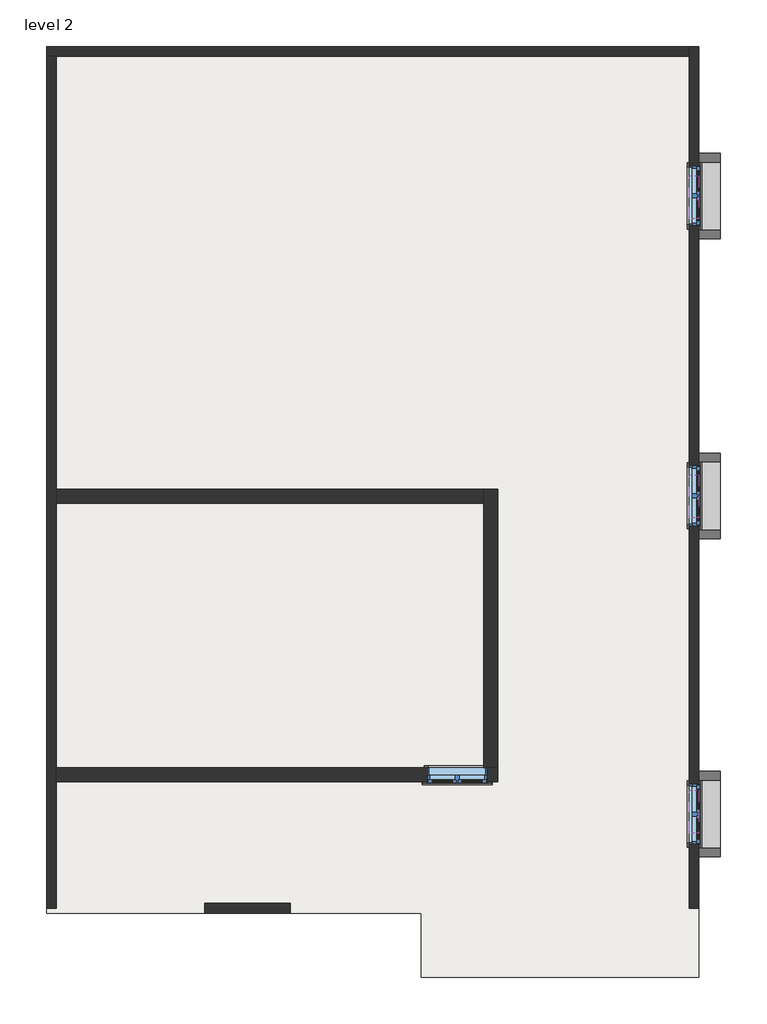
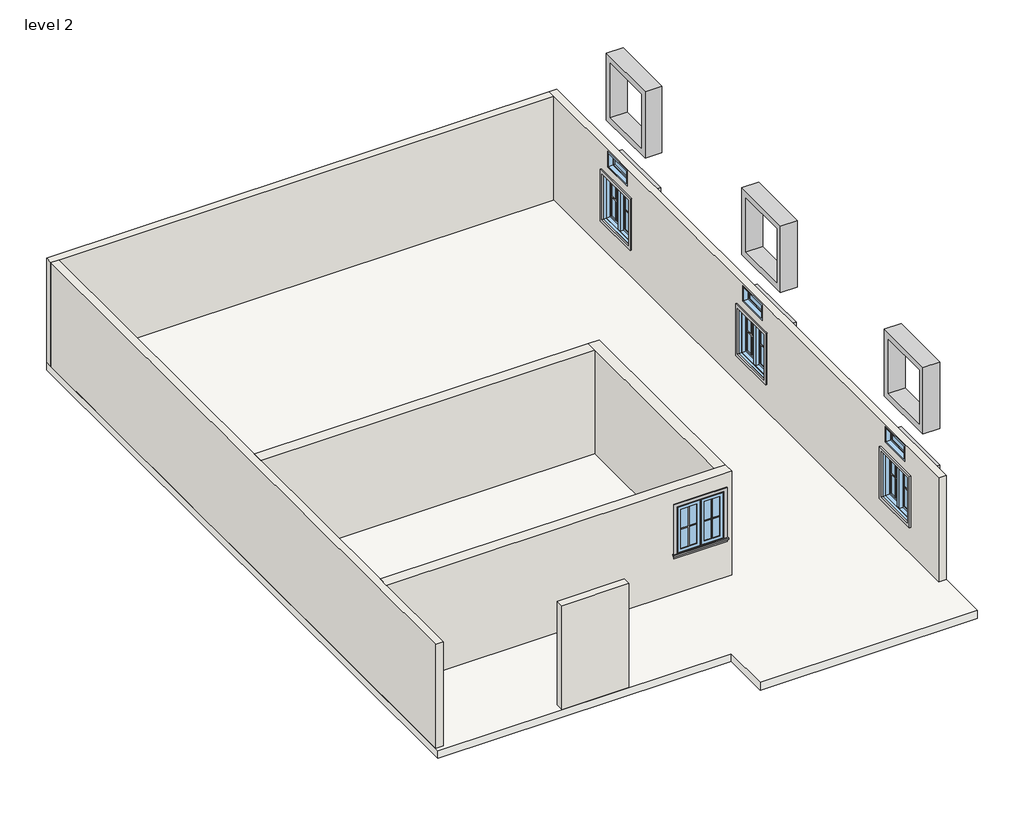
# One storey, incomplete: 16 proxies, 7 walls, 7 windows, 1 duct fitting, 1 slab.
"""IFC4 building model written with IfcOpenShell, lengths in millimetres."""

from ifc_helpers import new_model, si_unit, frame, origin, place, context, project, spatial, polyline, outline, extrude, faceted_brep, transform, mapped, element, save
from components import m_muntin_pattern_2x2_m_muntin_pattern_2x2_62480ac4, m_muntin_pattern_2x2_m_muntin_pattern_2x2_4fd78f17, m_trim_window_exterior_flat_with_sill_90d3a428, m_trim_window_interior_flat_picture_frame_6ca9b1f8, duct_fittings_2_duct_fittings_2_84becefd, m_fixed_0406_x_0610mm_8d3231a3, m_window_casement_double_850_x_900mm_0f766704, m_window_casement_double_850_x_900mm_77c4388a

model = new_model("IFC4")

# Units and contexts
model_context = context("Model", 3, world=origin())
ifc_project = project(units=[si_unit("LENGTHUNIT", "METRE", prefix="MILLI")], contexts=[model_context])

# Site, building, storey
site = spatial("IfcSite", under=ifc_project)
building = spatial("IfcBuilding", under=site)
storey = spatial("IfcBuildingStorey", under=building, Name="level 2", Elevation=5000.0)

# Proxies
placement = place(None, origin())
m_muntin_pattern_2x2_m_muntin_pattern_2x2_shape = m_muntin_pattern_2x2_m_muntin_pattern_2x2_62480ac4(model_context)
element("IfcBuildingElementProxy", 1, Name="M_Muntin Pattern_2x2 : M_Muntin Pattern_2x2", ObjectType="M_Muntin Pattern_2x2 : M_Muntin Pattern_2x2", at=placement, inside=storey, context=model_context, shape_type="MappedRepresentation", body=[
    mapped(m_muntin_pattern_2x2_m_muntin_pattern_2x2_shape, transform((-5582.3542042, -3112.6046146, 5837.792842), x_axis=(-1.0, 0.0, 0.0), y_axis=(0.0, -1.0, 0.0), z_axis=(0.0, 0.0, 1.0))),
])
element("IfcBuildingElementProxy", 2, Name="M_Muntin Pattern_2x2 : M_Muntin Pattern_2x2", ObjectType="M_Muntin Pattern_2x2 : M_Muntin Pattern_2x2", at=placement, inside=storey, context=model_context, shape_type="MappedRepresentation", body=[
    mapped(m_muntin_pattern_2x2_m_muntin_pattern_2x2_shape, transform((-2362.9917042, -3370.6171146, 5642.7567455), x_axis=(0.0, -1.0, 0.0), y_axis=(1.0, 0.0, 0.0), z_axis=(0.0, 0.0, 1.0))),
])
element("IfcBuildingElementProxy", 3, Name="M_Muntin Pattern_2x2 : M_Muntin Pattern_2x2", ObjectType="M_Muntin Pattern_2x2 : M_Muntin Pattern_2x2", at=placement, inside=storey, context=model_context, shape_type="MappedRepresentation", body=[
    mapped(m_muntin_pattern_2x2_m_muntin_pattern_2x2_shape, transform((-2362.9917042, 1160.7078854, 5642.7567455), x_axis=(0.0, -1.0, 0.0), y_axis=(1.0, 0.0, 0.0), z_axis=(0.0, 0.0, 1.0))),
])
element("IfcBuildingElementProxy", 4, Name="M_Muntin Pattern_2x2 : M_Muntin Pattern_2x2", ObjectType="M_Muntin Pattern_2x2 : M_Muntin Pattern_2x2", at=placement, inside=storey, context=model_context, shape_type="MappedRepresentation", body=[
    mapped(m_muntin_pattern_2x2_m_muntin_pattern_2x2_shape, transform((-2362.9917042, 5427.9078854, 5642.7567455), x_axis=(0.0, -1.0, 0.0), y_axis=(1.0, 0.0, 0.0), z_axis=(0.0, 0.0, 1.0))),
])
m_muntin_pattern_2x2_m_muntin_pattern_2x2_2_shape = m_muntin_pattern_2x2_m_muntin_pattern_2x2_4fd78f17(model_context)
element("IfcBuildingElementProxy", 5, Name="M_Muntin Pattern_2x2 : M_Muntin Pattern_2x2", ObjectType="M_Muntin Pattern_2x2 : M_Muntin Pattern_2x2", at=placement, inside=storey, context=model_context, shape_type="MappedRepresentation", body=[
    mapped(m_muntin_pattern_2x2_m_muntin_pattern_2x2_2_shape, transform((-6004.1792042, -3112.6046146, 5837.792842), x_axis=(1.0, 0.0, 0.0), y_axis=(0.0, 1.0, 0.0), z_axis=(0.0, 0.0, 1.0))),
])
element("IfcBuildingElementProxy", 6, Name="M_Muntin Pattern_2x2 : M_Muntin Pattern_2x2", ObjectType="M_Muntin Pattern_2x2 : M_Muntin Pattern_2x2", at=placement, inside=storey, context=model_context, shape_type="MappedRepresentation", body=[
    mapped(m_muntin_pattern_2x2_m_muntin_pattern_2x2_2_shape, transform((-2362.9917042, -3792.4421146, 5642.7567455), x_axis=(0.0, 1.0, 0.0), y_axis=(-1.0, 0.0, 0.0), z_axis=(0.0, 0.0, 1.0))),
])
element("IfcBuildingElementProxy", 7, Name="M_Muntin Pattern_2x2 : M_Muntin Pattern_2x2", ObjectType="M_Muntin Pattern_2x2 : M_Muntin Pattern_2x2", at=placement, inside=storey, context=model_context, shape_type="MappedRepresentation", body=[
    mapped(m_muntin_pattern_2x2_m_muntin_pattern_2x2_2_shape, transform((-2362.9917042, 738.8828854, 5642.7567455), x_axis=(0.0, 1.0, 0.0), y_axis=(-1.0, 0.0, 0.0), z_axis=(0.0, 0.0, 1.0))),
])
element("IfcBuildingElementProxy", 8, Name="M_Muntin Pattern_2x2 : M_Muntin Pattern_2x2", ObjectType="M_Muntin Pattern_2x2 : M_Muntin Pattern_2x2", at=placement, inside=storey, context=model_context, shape_type="MappedRepresentation", body=[
    mapped(m_muntin_pattern_2x2_m_muntin_pattern_2x2_2_shape, transform((-2362.9917042, 5006.0828854, 5642.7567455), x_axis=(0.0, 1.0, 0.0), y_axis=(-1.0, 0.0, 0.0), z_axis=(0.0, 0.0, 1.0))),
])
m_trim_window_exterior_flat_with_sill_shape = m_trim_window_exterior_flat_with_sill_90d3a428(model_context)
element("IfcBuildingElementProxy", 9, Name="M_Trim-Window-Exterior-Flat : with Sill", ObjectType="M_Trim-Window-Exterior-Flat : with Sill", at=placement, inside=storey, context=model_context, shape_type="MappedRepresentation", body=[
    mapped(m_trim_window_exterior_flat_with_sill_shape, transform((-5793.2667042, -3122.1296146, 6667.942842), x_axis=(1.0, 0.0, 0.0), y_axis=(0.0, 0.0, 1.0), z_axis=(0.0, -1.0, 0.0))),
])
element("IfcBuildingElementProxy", 10, Name="M_Trim-Window-Exterior-Flat : with Sill", ObjectType="M_Trim-Window-Exterior-Flat : with Sill", at=placement, inside=storey, context=model_context, shape_type="MappedRepresentation", body=[
    mapped(m_trim_window_exterior_flat_with_sill_shape, transform((-2353.4667042, -3581.5296146, 6472.9067455), x_axis=(0.0, 1.0, 0.0), y_axis=(0.0, 0.0, 1.0), z_axis=(1.0, 0.0, 0.0))),
])
element("IfcBuildingElementProxy", 11, Name="M_Trim-Window-Exterior-Flat : with Sill", ObjectType="M_Trim-Window-Exterior-Flat : with Sill", at=placement, inside=storey, context=model_context, shape_type="MappedRepresentation", body=[
    mapped(m_trim_window_exterior_flat_with_sill_shape, transform((-2353.4667042, 949.7953854, 6472.9067455), x_axis=(0.0, 1.0, 0.0), y_axis=(0.0, 0.0, 1.0), z_axis=(1.0, 0.0, 0.0))),
])
element("IfcBuildingElementProxy", 12, Name="M_Trim-Window-Exterior-Flat : with Sill", ObjectType="M_Trim-Window-Exterior-Flat : with Sill", at=placement, inside=storey, context=model_context, shape_type="MappedRepresentation", body=[
    mapped(m_trim_window_exterior_flat_with_sill_shape, transform((-2353.4667042, 5216.9953854, 6472.9067455), x_axis=(0.0, 1.0, 0.0), y_axis=(0.0, 0.0, 1.0), z_axis=(1.0, 0.0, 0.0))),
])
m_trim_window_interior_flat_picture_frame_shape = m_trim_window_interior_flat_picture_frame_6ca9b1f8(model_context)
element("IfcBuildingElementProxy", 13, Name="M_Trim-Window-Interior-Flat : Picture Frame", ObjectType="M_Trim-Window-Interior-Flat : Picture Frame", at=placement, inside=storey, context=model_context, shape_type="MappedRepresentation", body=[
    mapped(m_trim_window_interior_flat_picture_frame_shape, transform((-5793.2667042, -2922.1296146, 6667.942842), x_axis=(-1.0, 0.0, 0.0), y_axis=(0.0, 0.0, 1.0), z_axis=(0.0, 1.0, 0.0))),
])
element("IfcBuildingElementProxy", 14, Name="M_Trim-Window-Interior-Flat : Picture Frame", ObjectType="M_Trim-Window-Interior-Flat : Picture Frame", at=placement, inside=storey, context=model_context, shape_type="MappedRepresentation", body=[
    mapped(m_trim_window_interior_flat_picture_frame_shape, transform((-2493.4667042, -3581.5296146, 6472.9067455), x_axis=(0.0, -1.0, 0.0), y_axis=(0.0, 0.0, 1.0), z_axis=(-1.0, 0.0, 0.0))),
])
element("IfcBuildingElementProxy", 15, Name="M_Trim-Window-Interior-Flat : Picture Frame", ObjectType="M_Trim-Window-Interior-Flat : Picture Frame", at=placement, inside=storey, context=model_context, shape_type="MappedRepresentation", body=[
    mapped(m_trim_window_interior_flat_picture_frame_shape, transform((-2493.4667042, 949.7953854, 6472.9067455), x_axis=(0.0, -1.0, 0.0), y_axis=(0.0, 0.0, 1.0), z_axis=(-1.0, 0.0, 0.0))),
])
element("IfcBuildingElementProxy", 16, Name="M_Trim-Window-Interior-Flat : Picture Frame", ObjectType="M_Trim-Window-Interior-Flat : Picture Frame", at=placement, inside=storey, context=model_context, shape_type="MappedRepresentation", body=[
    mapped(m_trim_window_interior_flat_picture_frame_shape, transform((-2493.4667042, 5216.9953854, 6472.9067455), x_axis=(0.0, -1.0, 0.0), y_axis=(0.0, 0.0, 1.0), z_axis=(-1.0, 0.0, 0.0))),
])

# Duct fitting
duct_fittings_2_duct_fittings_2_shape = duct_fittings_2_duct_fittings_2_84becefd(model_context)
element("IfcDuctFitting", 17, ObjectType="Duct Fittings 2 : Duct Fittings 2", at=placement, inside=storey, context=model_context, shape_type="MappedRepresentation", body=[
    mapped(duct_fittings_2_duct_fittings_2_shape, transform((0.0, 0.0, 0.0), x_axis=(1.0, 0.0, 0.0), y_axis=(0.0, 1.0, 0.0), z_axis=(0.0, 0.0, 1.0))),
])

# Slab
element("IfcSlab", 18, ObjectType="Generic 150mm", at=placement, inside=storey, context=model_context, shape_type="SweptSolid", body=[
    extrude(outline(polyline([(-2353.4667042, 7341.0703854), (-2353.4667042, -5905.3296146), (-6306.9843842, -5905.3296146), (-6306.9843842, -4990.9296146), (-11637.4667042, -4990.9296146), (-11637.4667042, 7341.0703854), (-2353.4667042, 7341.0703854)])), frame((0.0, 0.0, 4850.0), z_axis=(0.0, 0.0, 1.0), x_axis=(1.0, 0.0, 0.0)), (0.0, 0.0, 1.0), 150.0),
])

# Walls
element("IfcWall", 19, ObjectType="Generic - 140mm Masonry", at=placement, inside=storey, context=model_context, shape_type="Brep", body=[
    faceted_brep([(-2353.4667042, -4920.9296146, 5000.0), (-2353.4667042, 7341.0703854, 5000.0), (-2353.4667042, 7341.0703854, 7000.0), (-2353.4667042, -4920.9296146, 7000.0), (-2353.4667042, -4006.5296146, 6472.9067455), (-2353.4667042, -3156.5296146, 6472.9067455), (-2353.4667042, -3156.5296146, 5572.9067455), (-2353.4667042, -4006.5296146, 5572.9067455), (-2353.4667042, 524.7953854, 6472.9067455), (-2353.4667042, 1374.7953854, 6472.9067455), (-2353.4667042, 1374.7953854, 5572.9067455), (-2353.4667042, 524.7953854, 5572.9067455), (-2353.4667042, 4791.9953854, 6472.9067455), (-2353.4667042, 5641.9953854, 6472.9067455), (-2353.4667042, 5641.9953854, 5572.9067455), (-2353.4667042, 4791.9953854, 5572.9067455), (-2353.4667042, -3244.5296146, 6674.2514163), (-2353.4667042, -3854.1296146, 6674.2514163), (-2353.4667042, -3854.1296146, 6979.0514163), (-2353.4667042, -3244.5296146, 6979.0514163), (-2353.4667042, 1244.9203854, 6663.0676988), (-2353.4667042, 635.3203854, 6663.0676988), (-2353.4667042, 635.3203854, 6967.8676988), (-2353.4667042, 1244.9203854, 6967.8676988), (-2353.4667042, 5499.2703854, 6665.4707754), (-2353.4667042, 4889.6703854, 6665.4707754), (-2353.4667042, 4889.6703854, 6970.2707754), (-2353.4667042, 5499.2703854, 6970.2707754), (-2493.4667042, -4920.9296146, 5000.0), (-2493.4667042, -4920.9296146, 7000.0), (-2493.4667042, 7201.0703854, 7000.0), (-2493.4667042, 7341.0703854, 7000.0), (-2493.4667042, 7341.0703854, 5000.0), (-2493.4667042, 7201.0703854, 5000.0), (-2493.4667042, -4006.5296146, 6472.9067455), (-2493.4667042, -4006.5296146, 5572.9067455), (-2493.4667042, -3156.5296146, 5572.9067455), (-2493.4667042, -3156.5296146, 6472.9067455), (-2493.4667042, 524.7953854, 6472.9067455), (-2493.4667042, 524.7953854, 5572.9067455), (-2493.4667042, 1374.7953854, 5572.9067455), (-2493.4667042, 1374.7953854, 6472.9067455), (-2493.4667042, 4791.9953854, 6472.9067455), (-2493.4667042, 4791.9953854, 5572.9067455), (-2493.4667042, 5641.9953854, 5572.9067455), (-2493.4667042, 5641.9953854, 6472.9067455), (-2493.4667042, -3244.5296146, 6674.2514163), (-2493.4667042, -3244.5296146, 6979.0514163), (-2493.4667042, -3854.1296146, 6979.0514163), (-2493.4667042, -3854.1296146, 6674.2514163), (-2493.4667042, 1244.9203854, 6663.0676988), (-2493.4667042, 1244.9203854, 6967.8676988), (-2493.4667042, 635.3203854, 6967.8676988), (-2493.4667042, 635.3203854, 6663.0676988), (-2493.4667042, 5499.2703854, 6665.4707754), (-2493.4667042, 5499.2703854, 6970.2707754), (-2493.4667042, 4889.6703854, 6970.2707754), (-2493.4667042, 4889.6703854, 6665.4707754)], [[[0, 1, 2, 3], [4, 5, 6, 7], [8, 9, 10, 11], [12, 13, 14, 15], [16, 17, 18, 19], [20, 21, 22, 23], [24, 25, 26, 27]], [[28, 29, 30, 31, 32, 33], [34, 35, 36, 37], [38, 39, 40, 41], [42, 43, 44, 45], [46, 47, 48, 49], [50, 51, 52, 53], [54, 55, 56, 57]], [[1, 0, 28, 33, 32]], [[3, 2, 31, 30, 29]], [[0, 3, 29, 28]], [[2, 1, 32, 31]], [[35, 34, 4, 7]], [[36, 35, 7, 6]], [[37, 36, 6, 5]], [[34, 37, 5, 4]], [[39, 38, 8, 11]], [[40, 39, 11, 10]], [[41, 40, 10, 9]], [[38, 41, 9, 8]], [[43, 42, 12, 15]], [[44, 43, 15, 14]], [[45, 44, 14, 13]], [[42, 45, 13, 12]], [[47, 46, 16, 19]], [[48, 47, 19, 18]], [[49, 48, 18, 17]], [[46, 49, 17, 16]], [[51, 50, 20, 23]], [[52, 51, 23, 22]], [[53, 52, 22, 21]], [[50, 53, 21, 20]], [[55, 54, 24, 27]], [[56, 55, 27, 26]], [[57, 56, 26, 25]], [[54, 57, 25, 24]]]),
])
element("IfcWall", 20, ObjectType="Generic - 140mm Masonry", at=placement, inside=storey, context=model_context, shape_type="Brep", body=[
    faceted_brep([(-2493.4667042, 7341.0703854, 5000.0), (-11637.4667042, 7341.0703854, 5000.0), (-11637.4667042, 7341.0703854, 7000.0), (-2493.4667042, 7341.0703854, 7000.0), (-2493.4667042, 7201.0703854, 5000.0), (-2493.4667042, 7201.0703854, 7000.0), (-11497.4667042, 7201.0703854, 7000.0), (-11637.4667042, 7201.0703854, 7000.0), (-11637.4667042, 7201.0703854, 5000.0), (-11497.4667042, 7201.0703854, 5000.0)], [[[0, 1, 2, 3]], [[4, 5, 6, 7, 8, 9]], [[1, 0, 4, 9, 8]], [[3, 2, 7, 6, 5]], [[0, 3, 5, 4]], [[2, 1, 8, 7]]]),
])
element("IfcWall", 21, ObjectType="Generic - 140mm Masonry", at=placement, inside=storey, context=model_context, shape_type="Brep", body=[
    faceted_brep([(-11637.4667042, 7201.0703854, 5000.0), (-11637.4667042, -4920.9296146, 5000.0), (-11637.4667042, -4920.9296146, 7000.0), (-11637.4667042, 7201.0703854, 7000.0), (-11497.4667042, 7201.0703854, 5000.0), (-11497.4667042, 7201.0703854, 7000.0), (-11497.4667042, 1040.2703854, 7000.0), (-11497.4667042, 840.2703854, 7000.0), (-11497.4667042, -2922.1296146, 7000.0), (-11497.4667042, -3122.1296146, 7000.0), (-11497.4667042, -4920.9296146, 7000.0), (-11497.4667042, -4920.9296146, 5000.0), (-11497.4667042, -3122.1296146, 5000.0), (-11497.4667042, -2922.1296146, 5000.0), (-11497.4667042, 840.2703854, 5000.0), (-11497.4667042, 1040.2703854, 5000.0)], [[[0, 1, 2, 3]], [[4, 5, 6, 7, 8, 9, 10, 11, 12, 13, 14, 15]], [[1, 0, 4, 15, 14, 13, 12, 11]], [[2, 1, 11, 10]], [[3, 2, 10, 9, 8, 7, 6, 5]], [[0, 3, 5, 4]]]),
])
element("IfcWall", 22, ObjectType="Generic - 140mm Masonry", at=placement, inside=storey, context=model_context, shape_type="SweptSolid", body=[
    extrude(outline(polyline([(-8166.2667042, -4990.9296146), (-9385.4667042, -4990.9296146), (-9385.4667042, -4850.9296146), (-8166.2667042, -4850.9296146), (-8166.2667042, -4990.9296146)])), frame((0.0, 0.0, 5000.0), z_axis=(0.0, 0.0, 1.0), x_axis=(1.0, 0.0, 0.0)), (0.0, 0.0, 1.0), 2000.0),
])
element("IfcWall", 23, ObjectType="Generic - 200mm", at=placement, inside=storey, context=model_context, shape_type="Brep", body=[
    faceted_brep([(-11497.4667042, -3122.1296146, 5000.0), (-5219.0667042, -3122.1296146, 5000.0), (-5219.0667042, -3122.1296146, 7000.0), (-11497.4667042, -3122.1296146, 7000.0), (-6218.2667042, -3122.1296146, 6667.942842), (-5368.2667042, -3122.1296146, 6667.942842), (-5368.2667042, -3122.1296146, 5767.942842), (-6218.2667042, -3122.1296146, 5767.942842), (-11497.4667042, -2922.1296146, 5000.0), (-11497.4667042, -2922.1296146, 7000.0), (-5419.0667042, -2922.1296146, 7000.0), (-5219.0667042, -2922.1296146, 7000.0), (-5219.0667042, -2922.1296146, 5000.0), (-5419.0667042, -2922.1296146, 5000.0), (-6218.2667042, -2922.1296146, 6667.942842), (-6218.2667042, -2922.1296146, 5767.942842), (-5368.2667042, -2922.1296146, 5767.942842), (-5368.2667042, -2922.1296146, 6667.942842)], [[[0, 1, 2, 3], [4, 5, 6, 7]], [[8, 9, 10, 11, 12, 13], [14, 15, 16, 17]], [[1, 0, 8, 13, 12]], [[3, 2, 11, 10, 9]], [[2, 1, 12, 11]], [[0, 3, 9, 8]], [[15, 14, 4, 7]], [[16, 15, 7, 6]], [[17, 16, 6, 5]], [[14, 17, 5, 4]]]),
])
element("IfcWall", 24, ObjectType="Generic - 200mm", at=placement, inside=storey, context=model_context, shape_type="Brep", body=[
    faceted_brep([(-5219.0667042, -2922.1296146, 5000.0), (-5219.0667042, 1040.2703854, 5000.0), (-5219.0667042, 1040.2703854, 7000.0), (-5219.0667042, -2922.1296146, 7000.0), (-5419.0667042, -2922.1296146, 5000.0), (-5419.0667042, -2922.1296146, 7000.0), (-5419.0667042, 840.2703854, 7000.0), (-5419.0667042, 1040.2703854, 7000.0), (-5419.0667042, 1040.2703854, 5000.0), (-5419.0667042, 840.2703854, 5000.0)], [[[0, 1, 2, 3]], [[4, 5, 6, 7, 8, 9]], [[1, 0, 4, 9, 8]], [[3, 2, 7, 6, 5]], [[0, 3, 5, 4]], [[2, 1, 8, 7]]]),
])
element("IfcWall", 25, ObjectType="Generic - 200mm", at=placement, inside=storey, context=model_context, shape_type="SweptSolid", body=[
    extrude(outline(polyline([(-11497.4667042, 1040.2703854), (-5419.0667042, 1040.2703854), (-5419.0667042, 840.2703854), (-11497.4667042, 840.2703854), (-11497.4667042, 1040.2703854)])), frame((0.0, 0.0, 5000.0), z_axis=(0.0, 0.0, 1.0), x_axis=(1.0, 0.0, 0.0)), (0.0, 0.0, 1.0), 2000.0),
])

# Windows
m_fixed_0406_x_0610mm_shape = m_fixed_0406_x_0610mm_8d3231a3(model_context)
element("IfcWindow", 26, ObjectType="M_Fixed : 0406 x 0610mm", at=placement, inside=storey, context=model_context, shape_type="MappedRepresentation", body=[
    mapped(m_fixed_0406_x_0610mm_shape, transform((-2436.4667042, -3549.3296146, 5759.2514163), x_axis=(0.0, -1.0, 0.0), y_axis=(1.0, 0.0, 0.0), z_axis=(0.0, 0.0, 1.0))),
])
element("IfcWindow", 27, ObjectType="M_Fixed : 0406 x 0610mm", at=placement, inside=storey, context=model_context, shape_type="MappedRepresentation", body=[
    mapped(m_fixed_0406_x_0610mm_shape, transform((-2436.4667042, 940.1203854, 5748.0676988), x_axis=(0.0, -1.0, 0.0), y_axis=(1.0, 0.0, 0.0), z_axis=(0.0, 0.0, 1.0))),
])
element("IfcWindow", 28, ObjectType="M_Fixed : 0406 x 0610mm", at=placement, inside=storey, context=model_context, shape_type="MappedRepresentation", body=[
    mapped(m_fixed_0406_x_0610mm_shape, transform((-2436.4667042, 5194.4703854, 5750.4707754), x_axis=(0.0, -1.0, 0.0), y_axis=(1.0, 0.0, 0.0), z_axis=(0.0, 0.0, 1.0))),
])
m_window_casement_double_850_x_900mm_shape = m_window_casement_double_850_x_900mm_0f766704(model_context)
element("IfcWindow", 29, ObjectType="M_Window-Casement-Double : 850 x 900mm", at=placement, inside=storey, context=model_context, shape_type="MappedRepresentation", body=[
    mapped(m_window_casement_double_850_x_900mm_shape, transform((-5793.2667042, -3022.1296146, 4867.942842), x_axis=(-1.0, 0.0, 0.0), y_axis=(0.0, -1.0, 0.0), z_axis=(0.0, 0.0, 1.0))),
])
m_window_casement_double_850_x_900mm_2_shape = m_window_casement_double_850_x_900mm_77c4388a(model_context)
element("IfcWindow", 30, ObjectType="M_Window-Casement-Double : 850 x 900mm", at=placement, inside=storey, context=model_context, shape_type="MappedRepresentation", body=[
    mapped(m_window_casement_double_850_x_900mm_2_shape, transform((-2423.4667042, -3581.5296146, 4672.9067455), x_axis=(0.0, -1.0, 0.0), y_axis=(1.0, 0.0, 0.0), z_axis=(0.0, 0.0, 1.0))),
])
element("IfcWindow", 31, ObjectType="M_Window-Casement-Double : 850 x 900mm", at=placement, inside=storey, context=model_context, shape_type="MappedRepresentation", body=[
    mapped(m_window_casement_double_850_x_900mm_2_shape, transform((-2423.4667042, 949.7953854, 4672.9067455), x_axis=(0.0, -1.0, 0.0), y_axis=(1.0, 0.0, 0.0), z_axis=(0.0, 0.0, 1.0))),
])
element("IfcWindow", 32, ObjectType="M_Window-Casement-Double : 850 x 900mm", at=placement, inside=storey, context=model_context, shape_type="MappedRepresentation", body=[
    mapped(m_window_casement_double_850_x_900mm_2_shape, transform((-2423.4667042, 5216.9953854, 4672.9067455), x_axis=(0.0, -1.0, 0.0), y_axis=(1.0, 0.0, 0.0), z_axis=(0.0, 0.0, 1.0))),
])

save(model, "model.ifc")

# Revit data of these elements
# Type "M_Muntin Pattern_2x2 : M_Muntin Pattern_2x2"
#   Width [instance default] = 3.937008 ft
#   Thickness = 0.041667 ft
#   Height [instance default] = 3.937008 ft
#   Distance = 0.0625 ft
#   Interior Material [instance default] = none
#   Exterior Material [instance default] = none
#   Default Elevation = 0
# Type "M_Trim-Window-Exterior-Flat : with Sill"
#   Trim Width = 0.19685 ft
#   Trim Thickness_Picture Frame = 0.098425 ft
#   Trim Thickness_with Sill = 0.0625 ft
#   Sill Thickness = 0.098425 ft
#   Opening Width [instance default] = 1.968504 ft
#   Opening Height [instance default] = 2.952756 ft
#   Default Elevation = 3.937008 ft
#   Sill = yes
#   Picture Frame = no
#   Trim Material [instance default] = none
# Type "M_Trim-Window-Interior-Flat : Picture Frame"
#   Trim Thickness_Picture Frame = 0.098425 ft
#   Trim Width = 0.19685 ft
#   Trim Thickness_with Sill = 0.065617 ft
#   Sill Thickness = 0.098425 ft
#   Opening Width [instance default] = 1.968504 ft
#   Opening Height [instance default] = 2.952756 ft
#   Default Elevation = 3.937008 ft
#   Sill = no
#   Picture Frame = yes
#   Trim Material [instance default] = none
# Type "Generic 150mm"
#   Function = 0
#   Layers, outside or top first: 0.492126 ft no material (function 1)
# Type "Generic - 140mm Masonry"
#   Layers, outside or top first: 0.459318 ft "Concrete Masonry Units" (function 1)
# Type "Generic - 200mm"
#   Layers, outside or top first: 0.656168 ft no material (function 1)
# Type "M_Fixed : 0406 x 0610mm"
#   Type Mark = "10"
#   Construction Type Id = "GSP4R"
#   Analytic Construction = "1/8 in Pilkington single glazing"
#   Visual Light Transmittance = 0.9
#   Thermal Resistance (R) = 0.271106 (m²·K)/W
#   Solar Heat Gain Coefficient = 0.78
#   Heat Transfer Coefficient (U) = 3.6886 W/(m²·K)
#   Height = 1 ft
#   Default Sill Height = 3.001969 ft
#   Width = 2 ft
#   Window Inset = 0.062336 ft
#   Define Thermal Properties by = 1
#   Define Thermal Properties by = 1
#   Frame Exterior Material = Sash
#   Frame Interior Material = Sash
#   Glass Pane Material = Glass
#   Sash = Sash
#   Wall Closure = (empty or 0)
# Type "M_Window-Casement-Double : 850 x 900mm"
#   Type Mark = "23"
#   Fire Rating = "0.5h"
#   Assembly Code = "B2020100"
#   Analytic Construction = "Double glazing - domestic"
#   Frame Extension [instance default] = 0.020833 ft
#   Window Inset [instance default] = 0 ft
#   Wall Thickness [instance default] = 0.492126 ft
#   Interior Wall Closure [instance default] = 0.179626 ft
#   Half Width = 1.394357 ft
#   Visual Light Transmittance = 0.81
#   Thermal Resistance (R) = 0.319569 (m²·K)/W
#   Solar Heat Gain Coefficient = 0.76
#   Rough Width = 2.837927 ft
#   Rough Height = 3.001969 ft
#   Height = 2.952756 ft
#   Heat Transfer Coefficient (U) = 3.12929 W/(m²·K)
#   Exterior Wall Closure [instance default] = 0.104331 ft
#   Extension Jamb [instance default] = 0.179626 ft
#   Default Sill Height = 2.952756 ft
#   Width = 2.788714 ft
#   Define Thermal Properties by = 0
#   Muntin Visibility = yes
#   Interior Trim Visibility [instance default] = yes
#   Exterior Trim Visibility [instance default] = yes
#   Extension Jamb Visibility [instance default] = yes
#   Interior Trim Material = Wood - Stained
#   Muntin Pattern = M_Muntin Pattern_2x2 : M_Muntin Pattern_2x2
#   Interior Trim = M_Trim-Window-Interior-Flat : Picture Frame
#   Interior Frame Material = Wood - Stained
#   Glass Panel Material = Glass
#   Exterior Trim Material = Clad - White
#   Exterior Trim = M_Trim-Window-Exterior-Flat : with Sill
#   Exterior Frame Material = Clad - White
#   Wall Closure = (empty or 0)
# Elements 1, 2, 3, 4, 5, 6, 7, 8 (IfcBuildingElementProxy, "M_Muntin Pattern_2x2 : M_Muntin Pattern_2x2")
#   Width = 0.94644 ft
#   Height = 2.494423 ft
#   Interior Material = Wood - Stained
#   Exterior Material = Clad - White
#   Phase Created = New Construction
#   Materials on its faces: "Clad - White", "Wood - Stained"
# Elements 9, 10, 11, 12 (IfcBuildingElementProxy, "M_Trim-Window-Exterior-Flat : with Sill")
#   Opening Width = 2.788714 ft
#   Opening Height = 2.952756 ft
#   Trim Material = Clad - White
#   Phase Created = New Construction
#   Materials on its faces: "Clad - White"
# Elements 13, 14, 15, 16 (IfcBuildingElementProxy, "M_Trim-Window-Interior-Flat : Picture Frame")
#   Opening Width = 2.788714 ft
#   Opening Height = 2.952756 ft
#   Trim Material = Wood - Stained
#   Phase Created = New Construction
#   Materials on its faces: "Wood - Stained"
# Element 17 (IfcDuctFitting, "Duct Fittings 2 : Duct Fittings 2")
#   Phase Created = New Construction
#   Materials on its faces: "BB"
# Element 18 (IfcSlab, "Generic 150mm")
#   Height Offset From Level = 0 ft
#   Phase Created = New Construction
#   Materials on its faces: "Default Floor"
# Element 19 (IfcWall, "Generic - 140mm Masonry")
#   Top Offset = 0 ft
#   Base Offset = 0 ft
#   wall height = 6.56168 ft
#   Phase Created = New Construction
#   Base Constraint = level 2
#   Top Constraint = level 3
#   Materials on its faces: "Concrete Masonry Units", "Cherry", "YELLOW"
# Element 20 (IfcWall, "Generic - 140mm Masonry")
#   Top Offset = 0 ft
#   Base Offset = 0 ft
#   wall height = 6.56168 ft
#   Phase Created = New Construction
#   Base Constraint = level 2
#   Top Constraint = level 3
#   Materials on its faces: "Concrete Masonry Units", "PAINT", "Cherry"
# Element 21 (IfcWall, "Generic - 140mm Masonry")
#   Top Offset = 0 ft
#   Base Offset = 0 ft
#   wall height = 6.56168 ft
#   Phase Created = New Construction
#   Base Constraint = level 2
#   Top Constraint = level 3
#   Materials on its faces: "Concrete Masonry Units", "Cherry", "PAINT"
# Element 22 (IfcWall, "Generic - 140mm Masonry")
#   Top Offset = 6.56168 ft
#   Base Offset = 0 ft
#   wall height = 6.56168 ft
#   Phase Created = New Construction
#   Base Constraint = level 2
#   Top Constraint = level 2
#   Materials on its faces: "Concrete Masonry Units", "Clad - White"
# Elements 23, 24 (IfcWall, "Generic - 200mm")
#   Top Offset = 0 ft
#   Base Offset = 0 ft
#   Unconnected Height = 6.56168 ft
#   wall height = 6.56168 ft
#   Phase Created = New Construction
#   Base Constraint = level 2
#   Materials on its faces: "Default Wall", "PAINT"
# Element 25 (IfcWall, "Generic - 200mm")
#   Top Offset = 0 ft
#   Base Offset = 0 ft
#   Unconnected Height = 6.56168 ft
#   wall height = 6.56168 ft
#   Phase Created = New Construction
#   Base Constraint = level 2
#   Materials on its faces: "Default Wall"
# Element 26 (IfcWindow, "M_Fixed : 0406 x 0610mm")
#   Mark = "22"
#   Phase Created = New Construction
#   Materials on its faces: "Sash", "Glass"
# Element 27 (IfcWindow, "M_Fixed : 0406 x 0610mm")
#   Mark = "25"
#   Phase Created = New Construction
#   Materials on its faces: "Sash", "Glass"
# Element 28 (IfcWindow, "M_Fixed : 0406 x 0610mm")
#   Mark = "26"
#   Phase Created = New Construction
#   Materials on its faces: "Sash", "Glass"
# Element 29 (IfcWindow, "M_Window-Casement-Double : 850 x 900mm")
#   Mark = "14"
#   Window Inset = 0 ft
#   Interior Wall Closure = 0.179626 ft
#   Frame Extension = 0.020833 ft
#   Exterior Wall Closure = 0.104331 ft
#   Interior Trim Visibility = yes
#   Exterior Trim Visibility = yes
#   Phase Created = New Construction
#   Materials on its faces: "Wood - Stained", "Glass", "Clad - White"
# Element 30 (IfcWindow, "M_Window-Casement-Double : 850 x 900mm")
#   Mark = "16"
#   Window Inset = 0 ft
#   Interior Wall Closure = 0.179626 ft
#   Frame Extension = 0.020833 ft
#   Exterior Wall Closure = 0.104331 ft
#   Interior Trim Visibility = yes
#   Exterior Trim Visibility = yes
#   Phase Created = New Construction
#   Materials on its faces: "Wood - Stained", "Glass", "Clad - White"
# Element 31 (IfcWindow, "M_Window-Casement-Double : 850 x 900mm")
#   Mark = "17"
#   Window Inset = 0 ft
#   Interior Wall Closure = 0.179626 ft
#   Frame Extension = 0.020833 ft
#   Exterior Wall Closure = 0.104331 ft
#   Interior Trim Visibility = yes
#   Exterior Trim Visibility = yes
#   Phase Created = New Construction
#   Materials on its faces: "Wood - Stained", "Glass", "Clad - White"
# Element 32 (IfcWindow, "M_Window-Casement-Double : 850 x 900mm")
#   Mark = "18"
#   Window Inset = 0 ft
#   Interior Wall Closure = 0.179626 ft
#   Frame Extension = 0.020833 ft
#   Exterior Wall Closure = 0.104331 ft
#   Interior Trim Visibility = yes
#   Exterior Trim Visibility = yes
#   Phase Created = New Construction
#   Materials on its faces: "Wood - Stained", "Glass", "Clad - White"
# Materials
#   "Concrete Masonry Units": class "Masonry", colour RGB 181 181 181, transparency 0, Description = "Concrete masonry units", Cost = 0
#   "Sash": class "Wood", colour RGB 224 178 126, transparency 0, Cost = 0
#   "Glass": class "Glass", colour RGB 0 128 192, transparency 0.9, Description = "Soda Lime Glass", Cost = 0
#   "Wood - Stained": class "Wood", colour RGB 224 178 126, transparency 0, Cost = 0
#   "Clad - White": class "Wood", colour RGB 242 242 238, transparency 0, Cost = 0
#   "BB": class "Generic", colour RGB 24 76 198, transparency 0, Cost = 0
#   "Default Floor": colour RGB 127 127 127, transparency 0, Cost = 0
#   "Cherry": class "Wood", colour RGB 226 177 128, transparency 0, Description = "Prunus Serotina", Cost = 0
#   "YELLOW": class "Generic", colour RGB 255 255 0, transparency 0, Cost = 0
#   "PAINT": class "Generic", colour RGB 105 77 58, transparency 0, Cost = 0
#   "Default Wall": colour RGB 128 128 128, transparency 0, Cost = 0
